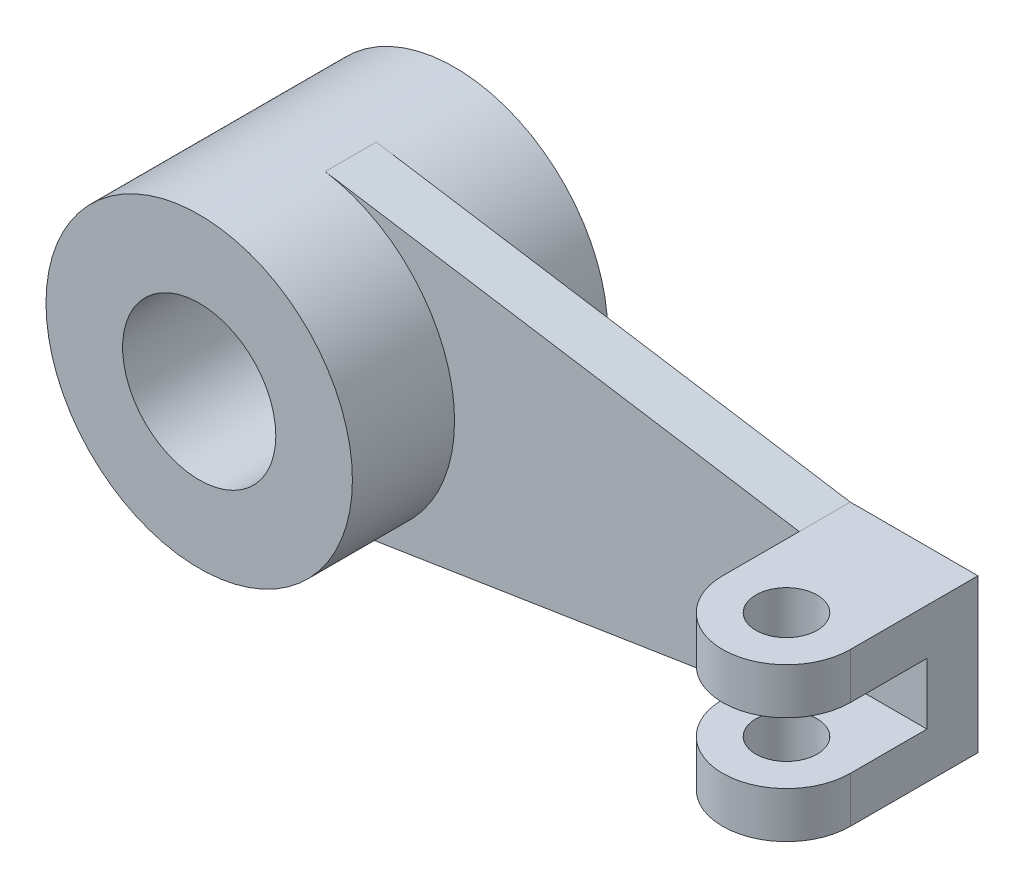
ISO-10303-21;
HEADER;
FILE_DESCRIPTION(('STEP AP214'),'2;1');
FILE_NAME('part.step','',(''),(''),'','','');
FILE_SCHEMA(('AUTOMOTIVE_DESIGN { 1 0 10303 214 1 1 1 1 }'));
ENDSEC;
DATA;
#1=APPLICATION_CONTEXT('core data for automotive mechanical design processes');
#2=APPLICATION_PROTOCOL_DEFINITION('international standard','automotive_design',2000,#1);
#3=PRODUCT_CONTEXT('',#1,'mechanical');
#4=PRODUCT('Part','Part','',(#3));
#5=PRODUCT_RELATED_PRODUCT_CATEGORY('part','',(#4));
#6=PRODUCT_DEFINITION_FORMATION('','',#4);
#7=PRODUCT_DEFINITION_CONTEXT('part definition',#1,'design');
#8=PRODUCT_DEFINITION('design','',#6,#7);
#9=PRODUCT_DEFINITION_SHAPE('','',#8);
#10=(LENGTH_UNIT() NAMED_UNIT(*) SI_UNIT(.MILLI.,.METRE.));
#11=(NAMED_UNIT(*) PLANE_ANGLE_UNIT() SI_UNIT($,.RADIAN.));
#12=(NAMED_UNIT(*) SI_UNIT($,.STERADIAN.) SOLID_ANGLE_UNIT());
#13=UNCERTAINTY_MEASURE_WITH_UNIT(LENGTH_MEASURE(1.E-05),#10,'distance_accuracy_value','');
#14=(GEOMETRIC_REPRESENTATION_CONTEXT(3) GLOBAL_UNCERTAINTY_ASSIGNED_CONTEXT((#13)) GLOBAL_UNIT_ASSIGNED_CONTEXT((#10,
#11,#12)) REPRESENTATION_CONTEXT('',''));
#15=CARTESIAN_POINT('',(0.,0.,0.));
#16=DIRECTION('',(0.,0.,1.));
#17=DIRECTION('',(1.,0.,0.));
#18=AXIS2_PLACEMENT_3D('',#15,#16,#17);
#19=CARTESIAN_POINT('',(0.,0.,5.));
#20=DIRECTION('',(0.,0.,1.));
#21=DIRECTION('',(1.,0.,0.));
#22=AXIS2_PLACEMENT_3D('',#19,#20,#21);
#23=PLANE('',#22);
#24=DIRECTION('',(0.,1.,0.));
#25=VECTOR('',#24,1.);
#26=CARTESIAN_POINT('',(122.5,15.,5.));
#27=LINE('',#26,#25);
#28=CARTESIAN_POINT('',(122.5,-5.99999999999999,5.));
#29=VERTEX_POINT('',#28);
#30=CARTESIAN_POINT('',(122.5,6.,5.));
#31=VERTEX_POINT('',#30);
#32=EDGE_CURVE('E141',#29,#31,#27,.T.);
#33=ORIENTED_EDGE('',*,*,#32,.T.);
#34=DIRECTION('',(1.,0.,0.));
#35=VECTOR('',#34,1.);
#36=CARTESIAN_POINT('',(97.5,5.99999999999999,5.));
#37=LINE('',#36,#35);
#38=CARTESIAN_POINT('',(97.5,5.99999999999999,5.));
#39=VERTEX_POINT('',#38);
#40=EDGE_CURVE('E127',#39,#31,#37,.T.);
#41=ORIENTED_EDGE('',*,*,#40,.F.);
#42=DIRECTION('',(0.,1.,0.));
#43=VECTOR('',#42,1.);
#44=CARTESIAN_POINT('',(97.5,5.99999999999999,5.));
#45=LINE('',#44,#43);
#46=CARTESIAN_POINT('',(97.5,15.,5.));
#47=VERTEX_POINT('',#46);
#48=EDGE_CURVE('E133',#39,#47,#45,.T.);
#49=ORIENTED_EDGE('',*,*,#48,.T.);
#50=DIRECTION('',(-0.987800769478854,0.155722958541715,0.));
#51=VECTOR('',#50,1.);
#52=CARTESIAN_POINT('',(4.67168875625145,29.6340230843656,5.));
#53=LINE('',#52,#51);
#54=CARTESIAN_POINT('',(4.67168875625145,29.6340230843656,5.));
#55=VERTEX_POINT('',#54);
#56=EDGE_CURVE('E195',#47,#55,#53,.T.);
#57=ORIENTED_EDGE('',*,*,#56,.T.);
#58=CARTESIAN_POINT('',(0.,0.,5.));
#59=DIRECTION('',(0.,0.,-1.));
#60=DIRECTION('',(1.,0.,0.));
#61=AXIS2_PLACEMENT_3D('',#58,#59,#60);
#62=CIRCLE('',#61,30.);
#63=CARTESIAN_POINT('',(4.67168875625145,-29.6340230843656,5.));
#64=VERTEX_POINT('',#63);
#65=EDGE_CURVE('E191',#55,#64,#62,.T.);
#66=ORIENTED_EDGE('',*,*,#65,.T.);
#67=DIRECTION('',(0.987800769478854,0.155722958541715,0.));
#68=VECTOR('',#67,1.);
#69=CARTESIAN_POINT('',(4.67168875625145,-29.6340230843656,5.));
#70=LINE('',#69,#68);
#71=CARTESIAN_POINT('',(97.5,-15.,5.));
#72=VERTEX_POINT('',#71);
#73=EDGE_CURVE('E189',#64,#72,#70,.T.);
#74=ORIENTED_EDGE('',*,*,#73,.T.);
#75=DIRECTION('',(0.,-1.,0.));
#76=VECTOR('',#75,1.);
#77=CARTESIAN_POINT('',(97.5,-5.99999999999999,5.));
#78=LINE('',#77,#76);
#79=CARTESIAN_POINT('',(97.5,-5.99999999999999,5.));
#80=VERTEX_POINT('',#79);
#81=EDGE_CURVE('E53',#80,#72,#78,.T.);
#82=ORIENTED_EDGE('',*,*,#81,.F.);
#83=DIRECTION('',(1.,0.,0.));
#84=VECTOR('',#83,1.);
#85=CARTESIAN_POINT('',(97.5,-5.99999999999999,5.));
#86=LINE('',#85,#84);
#87=EDGE_CURVE('E59',#80,#29,#86,.T.);
#88=ORIENTED_EDGE('',*,*,#87,.T.);
#89=EDGE_LOOP('',(#33,#41,#49,#57,#66,#74,#82,#88));
#90=FACE_BOUND('',#89,.T.);
#91=ADVANCED_FACE('F39',(#90),#23,.T.);
#92=CARTESIAN_POINT('',(0.,0.,25.));
#93=DIRECTION('',(0.,0.,1.));
#94=DIRECTION('',(1.,0.,0.));
#95=AXIS2_PLACEMENT_3D('',#92,#93,#94);
#96=PLANE('',#95);
#97=CARTESIAN_POINT('',(0.,0.,25.));
#98=DIRECTION('',(0.,0.,1.));
#99=DIRECTION('',(1.,0.,0.));
#100=AXIS2_PLACEMENT_3D('',#97,#98,#99);
#101=CIRCLE('',#100,30.);
#102=CARTESIAN_POINT('',(30.,0.,25.));
#103=VERTEX_POINT('',#102);
#104=EDGE_CURVE('E11',#103,#103,#101,.T.);
#105=ORIENTED_EDGE('',*,*,#104,.T.);
#106=EDGE_LOOP('',(#105));
#107=FACE_BOUND('',#106,.T.);
#108=CARTESIAN_POINT('',(0.,0.,25.));
#109=DIRECTION('',(0.,0.,1.));
#110=DIRECTION('',(1.,0.,0.));
#111=AXIS2_PLACEMENT_3D('',#108,#109,#110);
#112=CIRCLE('',#111,15.);
#113=CARTESIAN_POINT('',(15.,0.,25.));
#114=VERTEX_POINT('',#113);
#115=EDGE_CURVE('E227',#114,#114,#112,.T.);
#116=ORIENTED_EDGE('',*,*,#115,.F.);
#117=EDGE_LOOP('',(#116));
#118=FACE_BOUND('',#117,.T.);
#119=ADVANCED_FACE('F253',(#107,#118),#96,.T.);
#120=CARTESIAN_POINT('',(0.,0.,-25.));
#121=DIRECTION('',(0.,0.,1.));
#122=DIRECTION('',(1.,0.,0.));
#123=AXIS2_PLACEMENT_3D('',#120,#121,#122);
#124=PLANE('',#123);
#125=CARTESIAN_POINT('',(0.,0.,-25.));
#126=DIRECTION('',(0.,0.,1.));
#127=DIRECTION('',(1.,0.,0.));
#128=AXIS2_PLACEMENT_3D('',#125,#126,#127);
#129=CIRCLE('',#128,30.);
#130=CARTESIAN_POINT('',(30.,0.,-25.));
#131=VERTEX_POINT('',#130);
#132=EDGE_CURVE('E43',#131,#131,#129,.T.);
#133=ORIENTED_EDGE('',*,*,#132,.F.);
#134=EDGE_LOOP('',(#133));
#135=FACE_BOUND('',#134,.T.);
#136=CARTESIAN_POINT('',(0.,0.,-25.));
#137=DIRECTION('',(0.,0.,1.));
#138=DIRECTION('',(1.,0.,0.));
#139=AXIS2_PLACEMENT_3D('',#136,#137,#138);
#140=CIRCLE('',#139,15.);
#141=CARTESIAN_POINT('',(15.,0.,-25.));
#142=VERTEX_POINT('',#141);
#143=EDGE_CURVE('E226',#142,#142,#140,.T.);
#144=ORIENTED_EDGE('',*,*,#143,.T.);
#145=EDGE_LOOP('',(#144));
#146=FACE_BOUND('',#145,.T.);
#147=ADVANCED_FACE('F234',(#135,#146),#124,.F.);
#148=CARTESIAN_POINT('',(0.,0.,25.));
#149=DIRECTION('',(0.,0.,-1.));
#150=DIRECTION('',(-1.,0.,0.));
#151=AXIS2_PLACEMENT_3D('',#148,#149,#150);
#152=CYLINDRICAL_SURFACE('',#151,30.);
#153=DIRECTION('',(0.,0.,-1.));
#154=VECTOR('',#153,1.);
#155=CARTESIAN_POINT('',(4.67168875625144,-29.6340230843656,5.));
#156=LINE('',#155,#154);
#157=CARTESIAN_POINT('',(4.67168875625145,-29.6340230843656,-5.));
#158=VERTEX_POINT('',#157);
#159=EDGE_CURVE('E197',#64,#158,#156,.T.);
#160=ORIENTED_EDGE('',*,*,#159,.F.);
#161=ORIENTED_EDGE('',*,*,#65,.F.);
#162=DIRECTION('',(0.,0.,-1.));
#163=VECTOR('',#162,1.);
#164=CARTESIAN_POINT('',(4.67168875625145,29.6340230843656,5.));
#165=LINE('',#164,#163);
#166=CARTESIAN_POINT('',(4.67168875625145,29.6340230843656,-5.));
#167=VERTEX_POINT('',#166);
#168=EDGE_CURVE('E215',#55,#167,#165,.T.);
#169=ORIENTED_EDGE('',*,*,#168,.T.);
#170=CARTESIAN_POINT('',(0.,0.,-5.));
#171=DIRECTION('',(0.,0.,-1.));
#172=DIRECTION('',(1.,0.,0.));
#173=AXIS2_PLACEMENT_3D('',#170,#171,#172);
#174=CIRCLE('',#173,30.);
#175=EDGE_CURVE('E190',#167,#158,#174,.T.);
#176=ORIENTED_EDGE('',*,*,#175,.T.);
#177=EDGE_LOOP('',(#160,#161,#169,#176));
#178=FACE_BOUND('',#177,.T.);
#179=ORIENTED_EDGE('',*,*,#104,.F.);
#180=EDGE_LOOP('',(#179));
#181=FACE_BOUND('',#180,.T.);
#182=ORIENTED_EDGE('',*,*,#132,.T.);
#183=EDGE_LOOP('',(#182));
#184=FACE_BOUND('',#183,.T.);
#185=ADVANCED_FACE('F41',(#178,#181,#184),#152,.T.);
#186=CARTESIAN_POINT('',(0.,0.,25.));
#187=DIRECTION('',(0.,0.,-1.));
#188=DIRECTION('',(-1.,0.,0.));
#189=AXIS2_PLACEMENT_3D('',#186,#187,#188);
#190=CYLINDRICAL_SURFACE('',#189,15.);
#191=ORIENTED_EDGE('',*,*,#115,.T.);
#192=EDGE_LOOP('',(#191));
#193=FACE_BOUND('',#192,.T.);
#194=ORIENTED_EDGE('',*,*,#143,.F.);
#195=EDGE_LOOP('',(#194));
#196=FACE_BOUND('',#195,.T.);
#197=ADVANCED_FACE('F233',(#193,#196),#190,.F.);
#198=CARTESIAN_POINT('',(4.67168875625145,-29.6340230843656,5.));
#199=DIRECTION('',(-0.155722958541715,0.987800769478854,0.));
#200=DIRECTION('',(-0.987800769478854,-0.155722958541715,0.));
#201=AXIS2_PLACEMENT_3D('',#198,#199,#200);
#202=PLANE('',#201);
#203=DIRECTION('',(0.987800769478854,0.155722958541715,0.));
#204=VECTOR('',#203,1.);
#205=CARTESIAN_POINT('',(4.67168875625145,-29.6340230843656,-5.));
#206=LINE('',#205,#204);
#207=CARTESIAN_POINT('',(97.5,-15.,-5.));
#208=VERTEX_POINT('',#207);
#209=EDGE_CURVE('E181',#158,#208,#206,.T.);
#210=ORIENTED_EDGE('',*,*,#209,.T.);
#211=DIRECTION('',(0.,0.,-1.));
#212=VECTOR('',#211,1.);
#213=CARTESIAN_POINT('',(97.5,-15.,5.));
#214=LINE('',#213,#212);
#215=EDGE_CURVE('E224',#72,#208,#214,.T.);
#216=ORIENTED_EDGE('',*,*,#215,.F.);
#217=ORIENTED_EDGE('',*,*,#73,.F.);
#218=ORIENTED_EDGE('',*,*,#159,.T.);
#219=EDGE_LOOP('',(#210,#216,#217,#218));
#220=FACE_BOUND('',#219,.T.);
#221=ADVANCED_FACE('F240',(#220),#202,.F.);
#222=CARTESIAN_POINT('',(97.5,-15.,5.));
#223=DIRECTION('',(0.,1.,0.));
#224=DIRECTION('',(-1.,0.,0.));
#225=AXIS2_PLACEMENT_3D('',#222,#223,#224);
#226=PLANE('',#225);
#227=DIRECTION('',(1.,0.,0.));
#228=VECTOR('',#227,1.);
#229=CARTESIAN_POINT('',(97.5,-15.,-5.));
#230=LINE('',#229,#228);
#231=CARTESIAN_POINT('',(122.5,-15.,-5.));
#232=VERTEX_POINT('',#231);
#233=EDGE_CURVE('E199',#208,#232,#230,.T.);
#234=ORIENTED_EDGE('',*,*,#233,.T.);
#235=DIRECTION('',(0.,0.,-1.));
#236=VECTOR('',#235,1.);
#237=CARTESIAN_POINT('',(122.5,-15.,5.));
#238=LINE('',#237,#236);
#239=CARTESIAN_POINT('',(122.5,-15.,20.));
#240=VERTEX_POINT('',#239);
#241=EDGE_CURVE('E219',#240,#232,#238,.T.);
#242=ORIENTED_EDGE('',*,*,#241,.F.);
#243=CARTESIAN_POINT('',(110.,-15.,20.));
#244=DIRECTION('',(0.,-1.,0.));
#245=DIRECTION('',(1.,0.,0.));
#246=AXIS2_PLACEMENT_3D('',#243,#244,#245);
#247=CIRCLE('',#246,12.5);
#248=CARTESIAN_POINT('',(97.5,-15.,20.));
#249=VERTEX_POINT('',#248);
#250=EDGE_CURVE('E162',#240,#249,#247,.T.);
#251=ORIENTED_EDGE('',*,*,#250,.T.);
#252=DIRECTION('',(0.,0.,-1.));
#253=VECTOR('',#252,1.);
#254=CARTESIAN_POINT('',(97.5,-15.,5.));
#255=LINE('',#254,#253);
#256=EDGE_CURVE('E169',#249,#72,#255,.T.);
#257=ORIENTED_EDGE('',*,*,#256,.T.);
#258=ORIENTED_EDGE('',*,*,#215,.T.);
#259=EDGE_LOOP('',(#234,#242,#251,#257,#258));
#260=FACE_BOUND('',#259,.T.);
#261=CARTESIAN_POINT('',(110.,-15.,20.));
#262=DIRECTION('',(0.,-1.,0.));
#263=DIRECTION('',(1.,0.,0.));
#264=AXIS2_PLACEMENT_3D('',#261,#262,#263);
#265=CIRCLE('',#264,6.);
#266=CARTESIAN_POINT('',(116.,-15.,20.));
#267=VERTEX_POINT('',#266);
#268=EDGE_CURVE('E158',#267,#267,#265,.T.);
#269=ORIENTED_EDGE('',*,*,#268,.F.);
#270=EDGE_LOOP('',(#269));
#271=FACE_BOUND('',#270,.T.);
#272=ADVANCED_FACE('F245',(#260,#271),#226,.F.);
#273=CARTESIAN_POINT('',(122.5,15.,5.));
#274=DIRECTION('',(-1.,0.,0.));
#275=DIRECTION('',(0.,0.,1.));
#276=AXIS2_PLACEMENT_3D('',#273,#274,#275);
#277=PLANE('',#276);
#278=DIRECTION('',(0.,1.,0.));
#279=VECTOR('',#278,1.);
#280=CARTESIAN_POINT('',(122.5,15.,-5.));
#281=LINE('',#280,#279);
#282=CARTESIAN_POINT('',(122.5,15.,-5.));
#283=VERTEX_POINT('',#282);
#284=EDGE_CURVE('E205',#232,#283,#281,.T.);
#285=ORIENTED_EDGE('',*,*,#284,.T.);
#286=DIRECTION('',(0.,0.,-1.));
#287=VECTOR('',#286,1.);
#288=CARTESIAN_POINT('',(122.5,15.,5.));
#289=LINE('',#288,#287);
#290=CARTESIAN_POINT('',(122.5,15.,20.));
#291=VERTEX_POINT('',#290);
#292=EDGE_CURVE('E220',#291,#283,#289,.T.);
#293=ORIENTED_EDGE('',*,*,#292,.F.);
#294=DIRECTION('',(0.,1.,0.));
#295=VECTOR('',#294,1.);
#296=CARTESIAN_POINT('',(122.5,6.,20.));
#297=LINE('',#296,#295);
#298=CARTESIAN_POINT('',(122.5,6.,20.));
#299=VERTEX_POINT('',#298);
#300=EDGE_CURVE('E154',#299,#291,#297,.T.);
#301=ORIENTED_EDGE('',*,*,#300,.F.);
#302=DIRECTION('',(0.,0.,1.));
#303=VECTOR('',#302,1.);
#304=CARTESIAN_POINT('',(122.5,6.,5.));
#305=LINE('',#304,#303);
#306=EDGE_CURVE('E143',#31,#299,#305,.T.);
#307=ORIENTED_EDGE('',*,*,#306,.F.);
#308=ORIENTED_EDGE('',*,*,#32,.F.);
#309=DIRECTION('',(0.,0.,1.));
#310=VECTOR('',#309,1.);
#311=CARTESIAN_POINT('',(122.5,-6.,5.));
#312=LINE('',#311,#310);
#313=CARTESIAN_POINT('',(122.5,-6.,20.));
#314=VERTEX_POINT('',#313);
#315=EDGE_CURVE('E170',#29,#314,#312,.T.);
#316=ORIENTED_EDGE('',*,*,#315,.T.);
#317=DIRECTION('',(0.,-1.,0.));
#318=VECTOR('',#317,1.);
#319=CARTESIAN_POINT('',(122.5,-6.,20.));
#320=LINE('',#319,#318);
#321=EDGE_CURVE('E180',#314,#240,#320,.T.);
#322=ORIENTED_EDGE('',*,*,#321,.T.);
#323=ORIENTED_EDGE('',*,*,#241,.T.);
#324=EDGE_LOOP('',(#285,#293,#301,#307,#308,#316,#322,#323));
#325=FACE_BOUND('',#324,.T.);
#326=ADVANCED_FACE('F274',(#325),#277,.F.);
#327=CARTESIAN_POINT('',(97.5,15.,5.));
#328=DIRECTION('',(0.,-1.,0.));
#329=DIRECTION('',(1.,0.,0.));
#330=AXIS2_PLACEMENT_3D('',#327,#328,#329);
#331=PLANE('',#330);
#332=DIRECTION('',(-1.,0.,0.));
#333=VECTOR('',#332,1.);
#334=CARTESIAN_POINT('',(97.5,15.,-5.));
#335=LINE('',#334,#333);
#336=CARTESIAN_POINT('',(97.5,15.,-5.));
#337=VERTEX_POINT('',#336);
#338=EDGE_CURVE('E204',#283,#337,#335,.T.);
#339=ORIENTED_EDGE('',*,*,#338,.T.);
#340=DIRECTION('',(0.,0.,-1.));
#341=VECTOR('',#340,1.);
#342=CARTESIAN_POINT('',(97.5,15.,5.));
#343=LINE('',#342,#341);
#344=EDGE_CURVE('E212',#47,#337,#343,.T.);
#345=ORIENTED_EDGE('',*,*,#344,.F.);
#346=DIRECTION('',(0.,0.,-1.));
#347=VECTOR('',#346,1.);
#348=CARTESIAN_POINT('',(97.5,15.,5.));
#349=LINE('',#348,#347);
#350=CARTESIAN_POINT('',(97.5,15.,20.));
#351=VERTEX_POINT('',#350);
#352=EDGE_CURVE('E140',#351,#47,#349,.T.);
#353=ORIENTED_EDGE('',*,*,#352,.F.);
#354=CARTESIAN_POINT('',(110.,15.,20.));
#355=DIRECTION('',(0.,-1.,0.));
#356=DIRECTION('',(1.,0.,0.));
#357=AXIS2_PLACEMENT_3D('',#354,#355,#356);
#358=CIRCLE('',#357,12.5);
#359=EDGE_CURVE('E145',#291,#351,#358,.T.);
#360=ORIENTED_EDGE('',*,*,#359,.F.);
#361=ORIENTED_EDGE('',*,*,#292,.T.);
#362=EDGE_LOOP('',(#339,#345,#353,#360,#361));
#363=FACE_BOUND('',#362,.T.);
#364=CARTESIAN_POINT('',(110.,15.,20.));
#365=DIRECTION('',(0.,-1.,0.));
#366=DIRECTION('',(1.,0.,0.));
#367=AXIS2_PLACEMENT_3D('',#364,#365,#366);
#368=CIRCLE('',#367,6.);
#369=CARTESIAN_POINT('',(116.,15.,20.));
#370=VERTEX_POINT('',#369);
#371=EDGE_CURVE('E146',#370,#370,#368,.T.);
#372=ORIENTED_EDGE('',*,*,#371,.T.);
#373=EDGE_LOOP('',(#372));
#374=FACE_BOUND('',#373,.T.);
#375=ADVANCED_FACE('F271',(#363,#374),#331,.F.);
#376=CARTESIAN_POINT('',(4.67168875625145,29.6340230843656,5.));
#377=DIRECTION('',(-0.155722958541715,-0.987800769478854,0.));
#378=DIRECTION('',(0.987800769478854,-0.155722958541715,0.));
#379=AXIS2_PLACEMENT_3D('',#376,#377,#378);
#380=PLANE('',#379);
#381=DIRECTION('',(-0.987800769478854,0.155722958541715,0.));
#382=VECTOR('',#381,1.);
#383=CARTESIAN_POINT('',(4.67168875625145,29.6340230843656,-5.));
#384=LINE('',#383,#382);
#385=EDGE_CURVE('E206',#337,#167,#384,.T.);
#386=ORIENTED_EDGE('',*,*,#385,.T.);
#387=ORIENTED_EDGE('',*,*,#168,.F.);
#388=ORIENTED_EDGE('',*,*,#56,.F.);
#389=ORIENTED_EDGE('',*,*,#344,.T.);
#390=EDGE_LOOP('',(#386,#387,#388,#389));
#391=FACE_BOUND('',#390,.T.);
#392=ADVANCED_FACE('F270',(#391),#380,.F.);
#393=CARTESIAN_POINT('',(0.,0.,-5.));
#394=DIRECTION('',(0.,0.,1.));
#395=DIRECTION('',(1.,0.,0.));
#396=AXIS2_PLACEMENT_3D('',#393,#394,#395);
#397=PLANE('',#396);
#398=ORIENTED_EDGE('',*,*,#209,.F.);
#399=ORIENTED_EDGE('',*,*,#175,.F.);
#400=ORIENTED_EDGE('',*,*,#385,.F.);
#401=ORIENTED_EDGE('',*,*,#338,.F.);
#402=ORIENTED_EDGE('',*,*,#284,.F.);
#403=ORIENTED_EDGE('',*,*,#233,.F.);
#404=EDGE_LOOP('',(#398,#399,#400,#401,#402,#403));
#405=FACE_BOUND('',#404,.T.);
#406=ADVANCED_FACE('F263',(#405),#397,.F.);
#407=CARTESIAN_POINT('',(97.5,-5.99999999999999,5.));
#408=DIRECTION('',(-1.,0.,0.));
#409=DIRECTION('',(0.,-1.,0.));
#410=AXIS2_PLACEMENT_3D('',#407,#408,#409);
#411=PLANE('',#410);
#412=ORIENTED_EDGE('',*,*,#256,.F.);
#413=DIRECTION('',(0.,-1.,0.));
#414=VECTOR('',#413,1.);
#415=CARTESIAN_POINT('',(97.5,-5.99999999999999,20.));
#416=LINE('',#415,#414);
#417=CARTESIAN_POINT('',(97.5,-5.99999999999999,20.));
#418=VERTEX_POINT('',#417);
#419=EDGE_CURVE('E184',#418,#249,#416,.T.);
#420=ORIENTED_EDGE('',*,*,#419,.F.);
#421=DIRECTION('',(0.,0.,-1.));
#422=VECTOR('',#421,1.);
#423=CARTESIAN_POINT('',(97.5,-5.99999999999999,5.));
#424=LINE('',#423,#422);
#425=EDGE_CURVE('E173',#418,#80,#424,.T.);
#426=ORIENTED_EDGE('',*,*,#425,.T.);
#427=ORIENTED_EDGE('',*,*,#81,.T.);
#428=EDGE_LOOP('',(#412,#420,#426,#427));
#429=FACE_BOUND('',#428,.T.);
#430=ADVANCED_FACE('F266',(#429),#411,.T.);
#431=CARTESIAN_POINT('',(110.,-6.,20.));
#432=DIRECTION('',(0.,-1.,0.));
#433=DIRECTION('',(1.,0.,0.));
#434=AXIS2_PLACEMENT_3D('',#431,#432,#433);
#435=CYLINDRICAL_SURFACE('',#434,12.5);
#436=ORIENTED_EDGE('',*,*,#250,.F.);
#437=ORIENTED_EDGE('',*,*,#321,.F.);
#438=CARTESIAN_POINT('',(110.,-6.,20.));
#439=DIRECTION('',(0.,-1.,0.));
#440=DIRECTION('',(1.,0.,0.));
#441=AXIS2_PLACEMENT_3D('',#438,#439,#440);
#442=CIRCLE('',#441,12.5);
#443=EDGE_CURVE('E171',#314,#418,#442,.T.);
#444=ORIENTED_EDGE('',*,*,#443,.T.);
#445=ORIENTED_EDGE('',*,*,#419,.T.);
#446=EDGE_LOOP('',(#436,#437,#444,#445));
#447=FACE_BOUND('',#446,.T.);
#448=ADVANCED_FACE('F261',(#447),#435,.T.);
#449=CARTESIAN_POINT('',(110.,-6.,20.));
#450=DIRECTION('',(0.,-1.,0.));
#451=DIRECTION('',(1.,0.,0.));
#452=AXIS2_PLACEMENT_3D('',#449,#450,#451);
#453=PLANE('',#452);
#454=CARTESIAN_POINT('',(110.,-6.,20.));
#455=DIRECTION('',(0.,-1.,0.));
#456=DIRECTION('',(1.,0.,0.));
#457=AXIS2_PLACEMENT_3D('',#454,#455,#456);
#458=CIRCLE('',#457,6.);
#459=CARTESIAN_POINT('',(116.,-6.,20.));
#460=VERTEX_POINT('',#459);
#461=EDGE_CURVE('E159',#460,#460,#458,.T.);
#462=ORIENTED_EDGE('',*,*,#461,.T.);
#463=EDGE_LOOP('',(#462));
#464=FACE_BOUND('',#463,.T.);
#465=ORIENTED_EDGE('',*,*,#87,.F.);
#466=ORIENTED_EDGE('',*,*,#425,.F.);
#467=ORIENTED_EDGE('',*,*,#443,.F.);
#468=ORIENTED_EDGE('',*,*,#315,.F.);
#469=EDGE_LOOP('',(#465,#466,#467,#468));
#470=FACE_BOUND('',#469,.T.);
#471=ADVANCED_FACE('F289',(#464,#470),#453,.F.);
#472=CARTESIAN_POINT('',(110.,-6.,20.));
#473=DIRECTION('',(0.,-1.,0.));
#474=DIRECTION('',(1.,0.,0.));
#475=AXIS2_PLACEMENT_3D('',#472,#473,#474);
#476=CYLINDRICAL_SURFACE('',#475,6.);
#477=ORIENTED_EDGE('',*,*,#461,.F.);
#478=EDGE_LOOP('',(#477));
#479=FACE_BOUND('',#478,.T.);
#480=ORIENTED_EDGE('',*,*,#268,.T.);
#481=EDGE_LOOP('',(#480));
#482=FACE_BOUND('',#481,.T.);
#483=ADVANCED_FACE('F290',(#479,#482),#476,.F.);
#484=CARTESIAN_POINT('',(110.,6.,20.));
#485=DIRECTION('',(0.,1.,0.));
#486=DIRECTION('',(1.,0.,0.));
#487=AXIS2_PLACEMENT_3D('',#484,#485,#486);
#488=PLANE('',#487);
#489=ORIENTED_EDGE('',*,*,#40,.T.);
#490=ORIENTED_EDGE('',*,*,#306,.T.);
#491=CARTESIAN_POINT('',(110.,6.,20.));
#492=DIRECTION('',(0.,-1.,0.));
#493=DIRECTION('',(1.,0.,0.));
#494=AXIS2_PLACEMENT_3D('',#491,#492,#493);
#495=CIRCLE('',#494,12.5);
#496=CARTESIAN_POINT('',(97.5,5.99999999999999,20.));
#497=VERTEX_POINT('',#496);
#498=EDGE_CURVE('E126',#299,#497,#495,.T.);
#499=ORIENTED_EDGE('',*,*,#498,.T.);
#500=DIRECTION('',(0.,0.,-1.));
#501=VECTOR('',#500,1.);
#502=CARTESIAN_POINT('',(97.5,5.99999999999999,5.));
#503=LINE('',#502,#501);
#504=EDGE_CURVE('E122',#497,#39,#503,.T.);
#505=ORIENTED_EDGE('',*,*,#504,.T.);
#506=EDGE_LOOP('',(#489,#490,#499,#505));
#507=FACE_BOUND('',#506,.T.);
#508=CARTESIAN_POINT('',(110.,6.,20.));
#509=DIRECTION('',(0.,-1.,0.));
#510=DIRECTION('',(1.,0.,0.));
#511=AXIS2_PLACEMENT_3D('',#508,#509,#510);
#512=CIRCLE('',#511,6.);
#513=CARTESIAN_POINT('',(116.,6.,20.));
#514=VERTEX_POINT('',#513);
#515=EDGE_CURVE('E153',#514,#514,#512,.T.);
#516=ORIENTED_EDGE('',*,*,#515,.F.);
#517=EDGE_LOOP('',(#516));
#518=FACE_BOUND('',#517,.T.);
#519=ADVANCED_FACE('F124',(#507,#518),#488,.F.);
#520=CARTESIAN_POINT('',(110.,6.,20.));
#521=DIRECTION('',(0.,1.,0.));
#522=DIRECTION('',(-1.,0.,0.));
#523=AXIS2_PLACEMENT_3D('',#520,#521,#522);
#524=CYLINDRICAL_SURFACE('',#523,12.5);
#525=ORIENTED_EDGE('',*,*,#359,.T.);
#526=DIRECTION('',(0.,1.,0.));
#527=VECTOR('',#526,1.);
#528=CARTESIAN_POINT('',(97.5,5.99999999999999,20.));
#529=LINE('',#528,#527);
#530=EDGE_CURVE('E138',#497,#351,#529,.T.);
#531=ORIENTED_EDGE('',*,*,#530,.F.);
#532=ORIENTED_EDGE('',*,*,#498,.F.);
#533=ORIENTED_EDGE('',*,*,#300,.T.);
#534=EDGE_LOOP('',(#525,#531,#532,#533));
#535=FACE_BOUND('',#534,.T.);
#536=ADVANCED_FACE('F293',(#535),#524,.T.);
#537=CARTESIAN_POINT('',(97.5,5.99999999999999,5.));
#538=DIRECTION('',(1.,0.,0.));
#539=DIRECTION('',(0.,1.,0.));
#540=AXIS2_PLACEMENT_3D('',#537,#538,#539);
#541=PLANE('',#540);
#542=ORIENTED_EDGE('',*,*,#352,.T.);
#543=ORIENTED_EDGE('',*,*,#48,.F.);
#544=ORIENTED_EDGE('',*,*,#504,.F.);
#545=ORIENTED_EDGE('',*,*,#530,.T.);
#546=EDGE_LOOP('',(#542,#543,#544,#545));
#547=FACE_BOUND('',#546,.T.);
#548=ADVANCED_FACE('F135',(#547),#541,.F.);
#549=CARTESIAN_POINT('',(110.,6.,20.));
#550=DIRECTION('',(0.,1.,0.));
#551=DIRECTION('',(-1.,0.,0.));
#552=AXIS2_PLACEMENT_3D('',#549,#550,#551);
#553=CYLINDRICAL_SURFACE('',#552,6.);
#554=ORIENTED_EDGE('',*,*,#515,.T.);
#555=EDGE_LOOP('',(#554));
#556=FACE_BOUND('',#555,.T.);
#557=ORIENTED_EDGE('',*,*,#371,.F.);
#558=EDGE_LOOP('',(#557));
#559=FACE_BOUND('',#558,.T.);
#560=ADVANCED_FACE('F424',(#556,#559),#553,.F.);
#561=CLOSED_SHELL('',(#91,#119,#147,#185,#197,#221,#272,#326,#375,#392,#406,#430,#448,#471,#483,
#519,#536,#548,#560));
#562=MANIFOLD_SOLID_BREP('B2',#561);
#563=ADVANCED_BREP_SHAPE_REPRESENTATION('',(#18,#562),#14);
#564=SHAPE_DEFINITION_REPRESENTATION(#9,#563);
ENDSEC;
END-ISO-10303-21;
